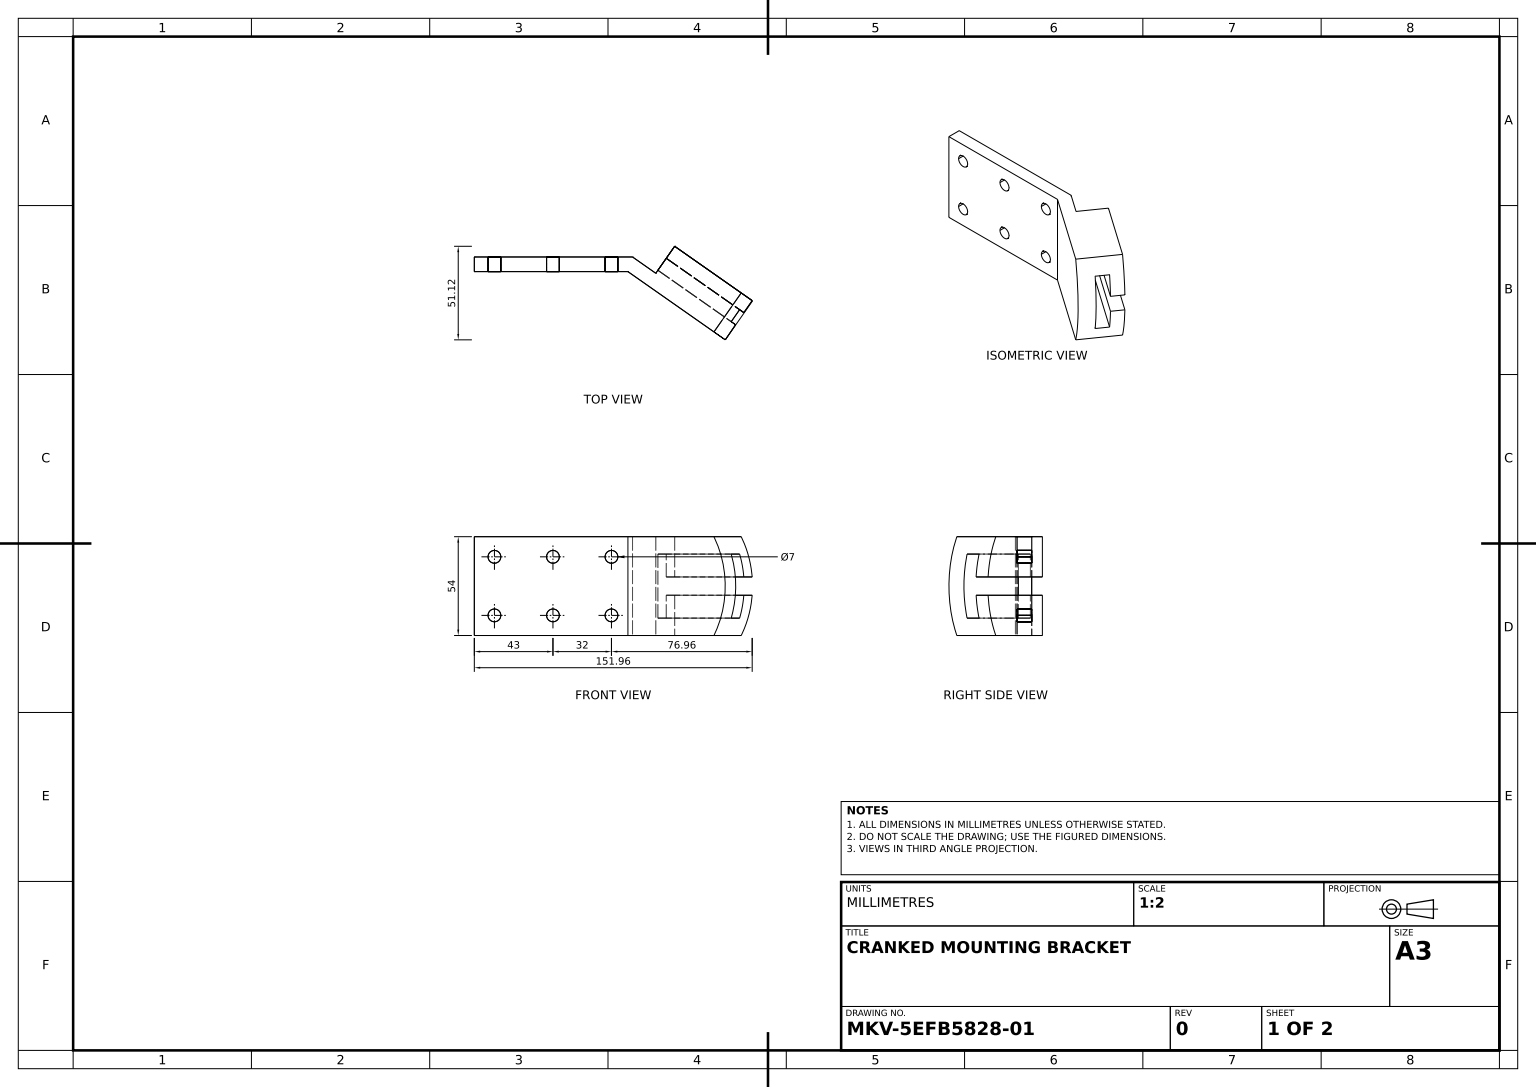
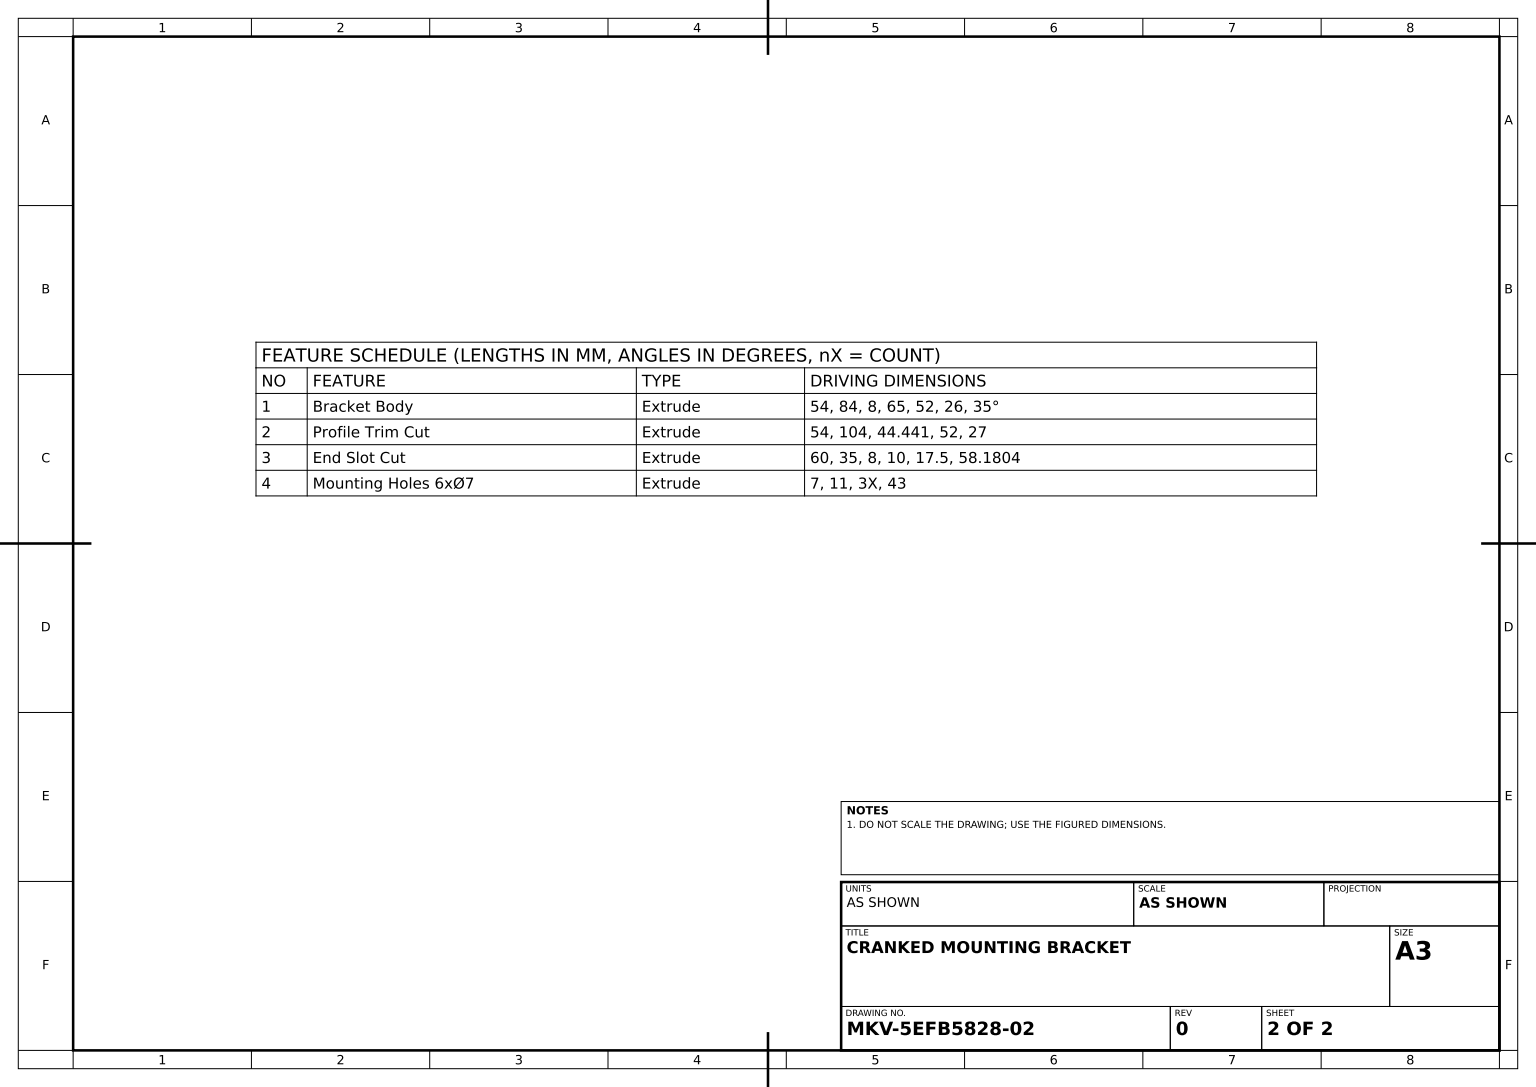
SolidWorks part; units mm, degrees
material "Plain Carbon Steel"
ref_plane "Front Plane" through (0, 0, 0) normal (0, 0, 1) x (1, 0, 0)
ref_plane "Top Plane" through (0, 0, 0) normal (0, 1, 0) x (1, 0, 0)
ref_plane "Right Plane" through (0, 0, 0) normal (1, 0, 0) x (0, 0, -1)
sketch "Bracket Profile Sketch" plane through (0, 0, 0) normal (0, 1, 0) x (1, 0, 0)
  line L0 (0, 0) -> (0, 8)
  line L1 (0, 8) -> (86.5224, 8)
  line L2 (86.5224, 8) -> (99.2376, -0.9033)
  line L7 (84, 0) -> (0, 0)
  line L8 (137.2449, -37.2825) -> (84, 0)
  line L9 (137.2449, -37.2825) -> (152.1579, -15.9845)
  line L10 (99.2376, -0.9033) -> (109.562, 13.8415)
  line L11 (152.1579, -15.9845) -> (109.562, 13.8415)
  dimension "D1" = 84
  dimension "D2" = 8
  dimension "D3" = 26
  dimension "D4" = 18
  dimension "D5" = 65
  dimension "D6" = 35
  dimension "D7" = 52
  dimension "D8" = 65
  dimension "D9" = 8
extrude "Bracket Body" add sketch "Bracket Profile Sketch" along normal mid plane 54
sketch "Profile Trim Sketch" plane through (42.5481, 0, -60.765) normal (0.5736, 0, -0.8192) x (-0.8192, 0, -0.5736)
  line L0 (-81.8088, 27) -> (-81.8088, -27) construction
  line L1 (-81.8088, 27) -> (-81.8088, -27) construction
  line L2 (-81.8088, 52) -> (-81.8088, -52)
  line L3 (-133.8088, 27) -> (-133.8088, -27)
  line L4 (-133.8088, -27) -> (-126.2497, -27)
  line L5 (-133.8088, -27) -> (-81.8088, -27) construction
  line L6 (-133.8088, 27) -> (-126.2497, 27)
  arc A0 (-81.8088, 52) -> (-81.8088, -52) centre (-81.8088, 0) ccw
  line M3 (-133.8088, -27) -> (-81.8088, -27)
  line M5 (-81.8088, 27) -> (-133.8088, 27)
  line M6 (-133.8088, 27) -> (-133.8088, -27)
  dimension "D1" = 104
  dimension "D2" = 44.441
  dimension "D3" = 52
  dimension "D4" = 27
  dimension "D5" = 54
extrude "Profile Trim Cut" cut sketch "Profile Trim Sketch" against normal blind 54 contours A0 M5 M6 | A0 L3 M3
ref_plane "Slot Sketch Plane" through (116.1629, 0, 81.3382) normal (-0.8192, 0, -0.5736) x (-0.5736, 0, 0.8192)
sketch "End Slot Sketch" plane through (116.1629, 0, 81.3382) normal (-0.8192, 0, -0.5736) x (-0.5736, 0, 0.8192)
  line L0 (-66.1804, -5) -> (-66.1804, -17.5)
  line L4 (-74.1804, 5) -> (-74.1804, -5)
  line L5 (-58.1804, 17.5) -> (-66.1804, 17.5)
  line L6 (-58.1804, 17.5) -> (-58.1804, -17.5)
  line L7 (-58.1804, -17.5) -> (-66.1804, -17.5)
  line L8 (-66.1804, 17.5) -> (-66.1804, 5)
  line L9 (-74.1804, -5) -> (-66.1804, -5)
  line L10 (-74.1804, -5) -> (-74.1804, 5)
  line L11 (-74.1804, 5) -> (-66.1804, 5)
  line L13 (-74.1804, -5) -> (-66.1804, 5) construction
  line L14 (-74.1804, 5) -> (-66.1804, -5) construction
  point P12 (-70.1804, 0)
  dimension "D1" = 35
  dimension "D2" = 8
  dimension "D3" = 17.5
  dimension "D4" = 8
  dimension "D5" = 8
  dimension "D6" = 10
  dimension "D7" = 58.1804
extrude "End Slot Cut" cut sketch "End Slot Sketch" along normal up to surface (60 mm away) contours L11 L4 L9 L0 L7 L6 L5 L8 up to face at (104.3998, 0, -6.4691)
sketch "Mounting Holes Sketch" plane through (0, 0, -8) normal (0, 0, -1) x (-1, 0, 0)
  line L0 (0, 27) -> (0, -27) construction
  line L1 (-86.5224, 27) -> (0, 27) construction
  line L2 (-86.5224, -27) -> (0, -27) construction
  circle A0 centre (-11, 16) radius 3.5
  circle A1 centre (-11, -16) radius 3.5
  circle A2 centre (-43, 16) radius 3.5
  circle A3 centre (-43, -16) radius 3.5
  circle A4 centre (-75, 16) radius 3.5
  circle A5 centre (-75, -16) radius 3.5
  dimension "D1" = 7
  dimension "D2" = 11
  dimension "D3" = 11
  dimension "D4" = 11
  dimension "D5" = 11
  dimension "D7" = 43
  dimension "D6" = 3
extrude "Mounting Holes 6xØ7" cut sketch "Mounting Holes Sketch" against normal up to surface (8 mm away) up to face at (42, 0, 0)
